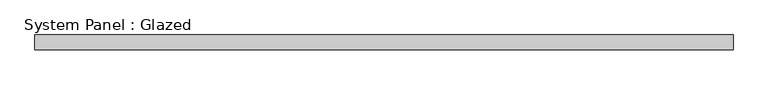
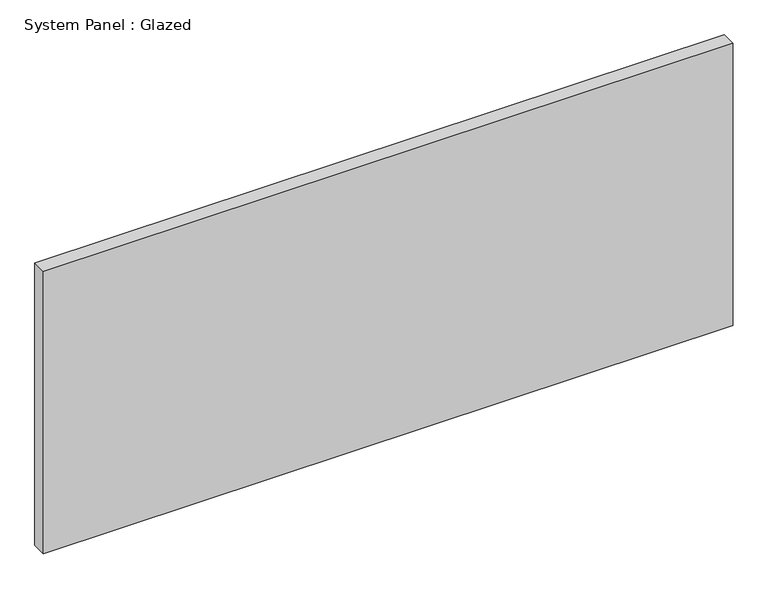
"""IFC4 building model written with IfcOpenShell, lengths in millimetres: plate geometry, System Panel : Glazed."""

from ifc_helpers import new_model, si_unit, origin, origin_with_axes, place, context, project, spatial, polyline, outline, extrude, source, transform, mapped, element, save


def system_panel_glazed_f2c52b8f(model_context):
    return source(origin(), model_context, "Body", "SweptSolid", [
        extrude(outline(polyline([(593.725, -44.45), (-593.725, -44.45), (-593.725, -19.05), (593.725, -19.05), (593.725, -44.45)])), origin_with_axes(), (0.0, 0.0, 1.0), 514.35),
    ])


if __name__ == "__main__":
    model = new_model("IFC4")
    model_context = context("Model", 3, world=origin())
    ifc_project = project(units=[si_unit("LENGTHUNIT", "METRE", prefix="MILLI")], contexts=[model_context])
    site = spatial("IfcSite", under=ifc_project)
    building = spatial("IfcBuilding", under=site)
    placement = place(None, origin())
    system_panel_glazed_shape = system_panel_glazed_f2c52b8f(model_context)
    element("IfcPlate", 1, ObjectType="System Panel : Glazed", at=placement, inside=building, context=model_context, shape_type="MappedRepresentation", body=[
        mapped(system_panel_glazed_shape, transform((0.0, 0.0, 0.0), x_axis=(1.0, 0.0, 0.0), y_axis=(0.0, 1.0, 0.0), z_axis=(0.0, 0.0, 1.0))),
    ])
    save(model, "model.ifc")

# Revit data of these elements
# Type "System Panel : Glazed"
#   Construction Type Id = "GSP4R"
#   Analytic Construction = "1/8 in Pilkington single glazing"
#   Visual Light Transmittance = 0.9
#   Solar Heat Gain Coefficient = 0.86
#   Heat Transfer Coefficient (U) = 1.18115 BTU/(h·ft²·°F)
# Element 1 (IfcPlate, "System Panel : Glazed")
#   Materials on its faces: "Glass"
# Materials
#   "Glass": class "Glass", colour RGB 0 128 192, transparency 0.75, Description = "Soda Lime Glass", Cost = 0
